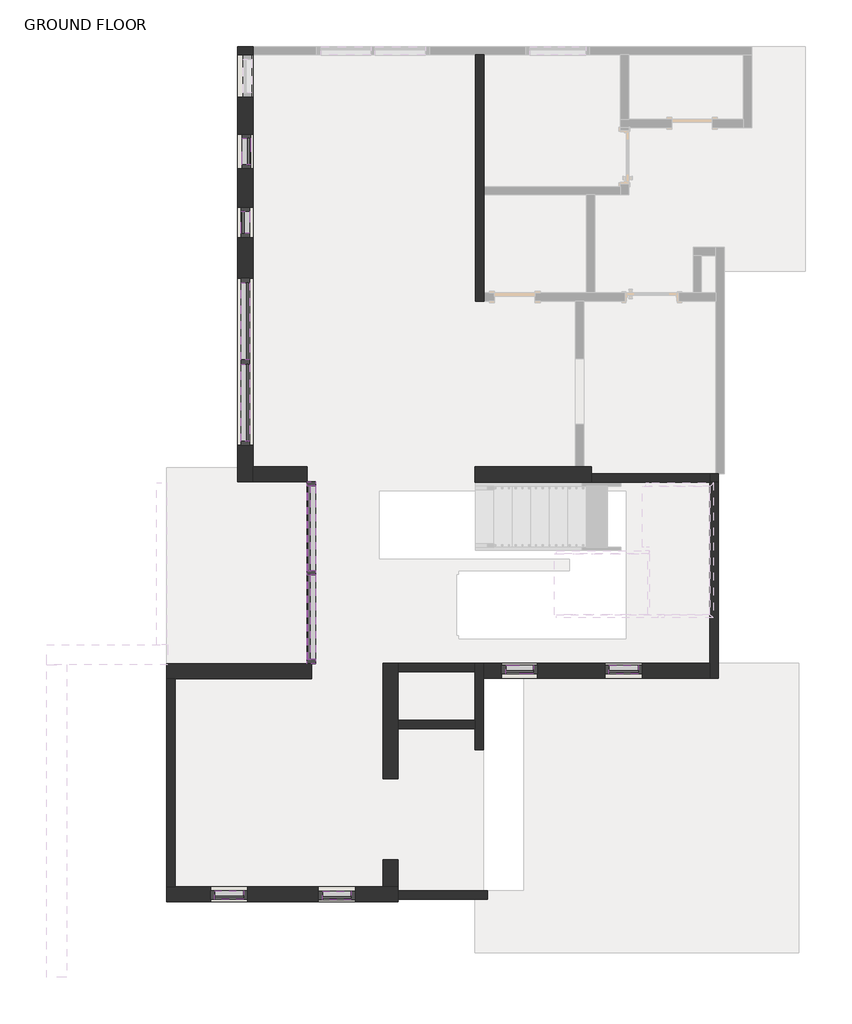
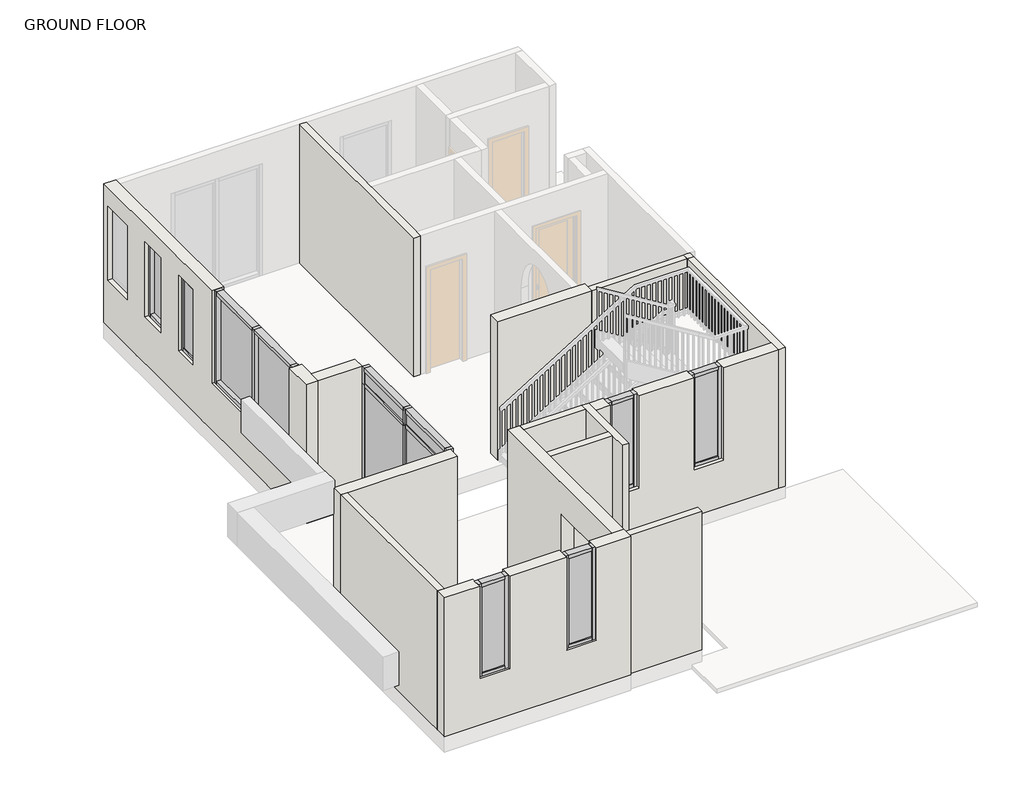
# One storey, part 1 of 3: 43 members, 16 walls, 12 plates.
"""IFC4 building model written with IfcOpenShell, lengths in millimetres."""

from ifc_helpers import new_model, si_unit, frame, origin, place, context, project, spatial, polyline, outline, extrude, faceted_brep, transform, mapped, element, save
from components import member_9ae880e2, member_2fc94954, member_ff9f2d30, member_7096a90e, member_6fb4a552, member_dc106669, member_69a911c1, member_2fae0574, member_d60e8053, member_28306602, member_d74100e1, member_f0fea5a5, member_f066cb84, member_ee409385, member_1c9aee36, member_0a8ab348, system_panel_glazed_1e1b7e15, system_panel_glazed_df80ca6a, system_panel_glazed_ba1f660c, system_panel_glazed_a5d4ee92, system_panel_glazed_c73a426b, system_panel_glazed_19c201ce, system_panel_glazed_de34110e, system_panel_glazed_f096bff0

model = new_model("IFC4")

# Units and contexts
model_context = context("Model", 3, world=origin())
ifc_project = project(units=[si_unit("LENGTHUNIT", "METRE", prefix="MILLI")], contexts=[model_context])

# Site, building, storey
site = spatial("IfcSite", under=ifc_project)
building = spatial("IfcBuilding", under=site)
storey = spatial("IfcBuildingStorey", under=building, Name="GROUND FLOOR", Elevation=304.8)

# Members
placement = place(None, origin())
member_shape = member_9ae880e2(model_context)
element("IfcMember", 1, ObjectType="Rectangular Mullion : 2.5\" x 5\" rectangular", at=placement, inside=storey, context=model_context, shape_type="MappedRepresentation", body=[
    mapped(member_shape, transform((-10742.5406521, -5304.9048674, 3048.0), x_axis=(0.0, 0.0, 1.0), y_axis=(1.0, 0.0, 0.0), z_axis=(0.0, 1.0, 0.0))),
])
element("IfcMember", 2, ObjectType="Rectangular Mullion : 2.5\" x 5\" rectangular", at=placement, inside=storey, context=model_context, shape_type="MappedRepresentation", body=[
    mapped(member_shape, transform((-10742.5406521, -6642.5105319, 3048.0), x_axis=(0.0, 0.0, 1.0), y_axis=(1.0, 0.0, 0.0), z_axis=(0.0, 1.0, 0.0))),
])
element("IfcMember", 3, ObjectType="Rectangular Mullion : 2.5\" x 5\" rectangular", at=placement, inside=storey, context=model_context, shape_type="MappedRepresentation", body=[
    mapped(member_shape, transform((-10742.5406521, -7916.6161964, 279.1402582), x_axis=(0.0, 0.0, -1.0), y_axis=(1.0, 0.0, 0.0), z_axis=(0.0, -1.0, 0.0))),
])
element("IfcMember", 4, ObjectType="Rectangular Mullion : 2.5\" x 5\" rectangular", at=placement, inside=storey, context=model_context, shape_type="MappedRepresentation", body=[
    mapped(member_shape, transform((-10742.5406521, -6579.0105319, 279.1402582), x_axis=(0.0, 0.0, -1.0), y_axis=(1.0, 0.0, 0.0), z_axis=(0.0, -1.0, 0.0))),
])
member_2_shape = member_2fc94954(model_context)
element("IfcMember", 5, ObjectType="Rectangular Mullion : 2.5\" x 5\" rectangular", at=placement, inside=storey, context=model_context, shape_type="MappedRepresentation", body=[
    mapped(member_2_shape, transform((-11735.5015106, -2244.2048674, 3048.0), x_axis=(0.0, 0.0, 1.0), y_axis=(1.0, 0.0, 0.0), z_axis=(0.0, 1.0, 0.0))),
])
element("IfcMember", 6, ObjectType="Rectangular Mullion : 2.5\" x 5\" rectangular", at=placement, inside=storey, context=model_context, shape_type="MappedRepresentation", body=[
    mapped(member_2_shape, transform((-11735.5015106, -3469.7548674, 3048.0), x_axis=(0.0, 0.0, 1.0), y_axis=(1.0, 0.0, 0.0), z_axis=(0.0, 1.0, 0.0))),
])
element("IfcMember", 7, ObjectType="Rectangular Mullion : 2.5\" x 5\" rectangular", at=placement, inside=storey, context=model_context, shape_type="MappedRepresentation", body=[
    mapped(member_2_shape, transform((-11735.5015106, -4631.8048674, 1219.2), x_axis=(0.0, 0.0, -1.0), y_axis=(1.0, 0.0, 0.0), z_axis=(0.0, -1.0, 0.0))),
])
element("IfcMember", 8, ObjectType="Rectangular Mullion : 2.5\" x 5\" rectangular", at=placement, inside=storey, context=model_context, shape_type="MappedRepresentation", body=[
    mapped(member_2_shape, transform((-11735.5015106, -3406.2548674, 1219.2), x_axis=(0.0, 0.0, -1.0), y_axis=(1.0, 0.0, 0.0), z_axis=(0.0, -1.0, 0.0))),
])
member_3_shape = member_ff9f2d30(model_context)
element("IfcMember", 9, ObjectType="Rectangular Mullion : 2.5\" x 5\" rectangular", at=placement, inside=storey, context=model_context, shape_type="MappedRepresentation", body=[
    mapped(member_3_shape, transform((-11735.5015106, -1171.7968948, 2709.2142793), x_axis=(0.0, 0.0, 1.0), y_axis=(1.0, 0.0, 0.0), z_axis=(0.0, 1.0, 0.0))),
])
element("IfcMember", 10, ObjectType="Rectangular Mullion : 2.5\" x 5\" rectangular", at=placement, inside=storey, context=model_context, shape_type="MappedRepresentation", body=[
    mapped(member_3_shape, transform((-11735.5015106, -1501.9968948, 1219.2), x_axis=(0.0, 0.0, -1.0), y_axis=(1.0, 0.0, 0.0), z_axis=(0.0, -1.0, 0.0))),
])
member_4_shape = member_7096a90e(model_context)
element("IfcMember", 11, ObjectType="Rectangular Mullion : 2.5\" x 5\" rectangular", at=placement, inside=storey, context=model_context, shape_type="MappedRepresentation", body=[
    mapped(member_4_shape, transform((-11716.8345465, -72.4462169, 2701.6314829), x_axis=(0.0, 0.0, 1.0), y_axis=(1.0, 0.0, 0.0), z_axis=(0.0, 1.0, 0.0))),
])
element("IfcMember", 12, ObjectType="Rectangular Mullion : 2.5\" x 5\" rectangular", at=placement, inside=storey, context=model_context, shape_type="MappedRepresentation", body=[
    mapped(member_4_shape, transform((-11716.8345465, -466.1462169, 1219.2), x_axis=(0.0, 0.0, -1.0), y_axis=(1.0, 0.0, 0.0), z_axis=(0.0, -1.0, 0.0))),
])
member_5_shape = member_6fb4a552(model_context)
element("IfcMember", 13, ObjectType="Rectangular Mullion : 2.5\" x 5\" rectangular", at=placement, inside=storey, context=model_context, shape_type="MappedRepresentation", body=[
    mapped(member_5_shape, transform((-6254.3081119, -8068.9864458, 3048.0), x_axis=(0.0, 0.0, 1.0), y_axis=(0.0, 1.0, 0.0), z_axis=(-1.0, 0.0, 0.0))),
])
element("IfcMember", 14, ObjectType="Rectangular Mullion : 2.5\" x 5\" rectangular", at=placement, inside=storey, context=model_context, shape_type="MappedRepresentation", body=[
    mapped(member_5_shape, transform((-5816.1581119, -8068.9864458, 1219.2), x_axis=(0.0, 0.0, -1.0), y_axis=(0.0, 1.0, 0.0), z_axis=(1.0, 0.0, 0.0))),
])
member_6_shape = member_dc106669(model_context)
element("IfcMember", 15, ObjectType="Rectangular Mullion : 2.5\" x 5\" rectangular", at=placement, inside=storey, context=model_context, shape_type="MappedRepresentation", body=[
    mapped(member_6_shape, transform((-7809.239759, -8066.9485269, 3048.0), x_axis=(0.0, 0.0, 1.0), y_axis=(0.0, 1.0, 0.0), z_axis=(-1.0, 0.0, 0.0))),
])
element("IfcMember", 16, ObjectType="Rectangular Mullion : 2.5\" x 5\" rectangular", at=placement, inside=storey, context=model_context, shape_type="MappedRepresentation", body=[
    mapped(member_6_shape, transform((-7396.489759, -8066.9485269, 1219.2), x_axis=(0.0, 0.0, -1.0), y_axis=(0.0, 1.0, 0.0), z_axis=(1.0, 0.0, 0.0))),
])
member_7_shape = member_69a911c1(model_context)
element("IfcMember", 17, ObjectType="Rectangular Mullion : 2.5\" x 5\" rectangular", at=placement, inside=storey, context=model_context, shape_type="MappedRepresentation", body=[
    mapped(member_7_shape, transform((-12196.3350942, -11462.667624, 3048.0), x_axis=(0.0, 0.0, 1.0), y_axis=(0.0, 1.0, 0.0), z_axis=(-1.0, 0.0, 0.0))),
])
element("IfcMember", 18, ObjectType="Rectangular Mullion : 2.5\" x 5\" rectangular", at=placement, inside=storey, context=model_context, shape_type="MappedRepresentation", body=[
    mapped(member_7_shape, transform((-10573.0486636, -11471.780526, 3048.0), x_axis=(0.0, 0.0, 1.0), y_axis=(0.0, 1.0, 0.0), z_axis=(-1.0, 0.0, 0.0))),
])
element("IfcMember", 19, ObjectType="Rectangular Mullion : 2.5\" x 5\" rectangular", at=placement, inside=storey, context=model_context, shape_type="MappedRepresentation", body=[
    mapped(member_7_shape, transform((-11764.5350942, -11462.667624, 1219.2), x_axis=(0.0, 0.0, -1.0), y_axis=(0.0, 1.0, 0.0), z_axis=(1.0, 0.0, 0.0))),
])
element("IfcMember", 20, ObjectType="Rectangular Mullion : 2.5\" x 5\" rectangular", at=placement, inside=storey, context=model_context, shape_type="MappedRepresentation", body=[
    mapped(member_7_shape, transform((-10141.2486636, -11471.780526, 1219.2), x_axis=(0.0, 0.0, -1.0), y_axis=(0.0, 1.0, 0.0), z_axis=(1.0, 0.0, 0.0))),
])
member_8_shape = member_2fae0574(model_context)
element("IfcMember", 21, ObjectType="Rectangular Mullion : 2.5\" x 5\" rectangular", at=placement, inside=storey, context=model_context, shape_type="MappedRepresentation", body=[
    mapped(member_8_shape, transform((-6317.8081119, -8068.9864458, 1219.2), x_axis=(-1.0, 0.0, 0.0), y_axis=(0.0, 1.0, 0.0), z_axis=(0.0, 0.0, -1.0))),
])
element("IfcMember", 22, ObjectType="Rectangular Mullion : 2.5\" x 5\" rectangular", at=placement, inside=storey, context=model_context, shape_type="MappedRepresentation", body=[
    mapped(member_8_shape, transform((-7872.739759, -8066.9485269, 1219.2), x_axis=(-1.0, 0.0, 0.0), y_axis=(0.0, 1.0, 0.0), z_axis=(0.0, 0.0, -1.0))),
])
element("IfcMember", 23, ObjectType="Rectangular Mullion : 2.5\" x 5\" rectangular", at=placement, inside=storey, context=model_context, shape_type="MappedRepresentation", body=[
    mapped(member_8_shape, transform((-12259.8350942, -11462.667624, 1219.2), x_axis=(-1.0, 0.0, 0.0), y_axis=(0.0, 1.0, 0.0), z_axis=(0.0, 0.0, -1.0))),
])
element("IfcMember", 24, ObjectType="Rectangular Mullion : 2.5\" x 5\" rectangular", at=placement, inside=storey, context=model_context, shape_type="MappedRepresentation", body=[
    mapped(member_8_shape, transform((-10636.5486636, -11471.780526, 1219.2), x_axis=(-1.0, 0.0, 0.0), y_axis=(0.0, 1.0, 0.0), z_axis=(0.0, 0.0, -1.0))),
])
element("IfcMember", 25, ObjectType="Rectangular Mullion : 2.5\" x 5\" rectangular", at=placement, inside=storey, context=model_context, shape_type="MappedRepresentation", body=[
    mapped(member_8_shape, transform((-5752.6581119, -8068.9864458, 3048.0), x_axis=(1.0, 0.0, 0.0), y_axis=(0.0, 1.0, 0.0), z_axis=(0.0, 0.0, 1.0))),
])
element("IfcMember", 26, ObjectType="Rectangular Mullion : 2.5\" x 5\" rectangular", at=placement, inside=storey, context=model_context, shape_type="MappedRepresentation", body=[
    mapped(member_8_shape, transform((-7332.989759, -8066.9485269, 3048.0), x_axis=(1.0, 0.0, 0.0), y_axis=(0.0, 1.0, 0.0), z_axis=(0.0, 0.0, 1.0))),
])
element("IfcMember", 27, ObjectType="Rectangular Mullion : 2.5\" x 5\" rectangular", at=placement, inside=storey, context=model_context, shape_type="MappedRepresentation", body=[
    mapped(member_8_shape, transform((-11701.0350942, -11462.667624, 3048.0), x_axis=(1.0, 0.0, 0.0), y_axis=(0.0, 1.0, 0.0), z_axis=(0.0, 0.0, 1.0))),
])
element("IfcMember", 28, ObjectType="Rectangular Mullion : 2.5\" x 5\" rectangular", at=placement, inside=storey, context=model_context, shape_type="MappedRepresentation", body=[
    mapped(member_8_shape, transform((-10077.7486636, -11471.780526, 3048.0), x_axis=(1.0, 0.0, 0.0), y_axis=(0.0, 1.0, 0.0), z_axis=(0.0, 0.0, 1.0))),
])
member_9_shape = member_d60e8053(model_context)
element("IfcMember", 29, ObjectType="Rectangular Mullion : 2.5\" x 5\" rectangular", at=placement, inside=storey, context=model_context, shape_type="MappedRepresentation", body=[
    mapped(member_9_shape, transform((-11735.5015106, -3438.0048674, 1219.2), x_axis=(0.0, 1.0, 0.0), y_axis=(1.0, 0.0, 0.0), z_axis=(0.0, 0.0, -1.0))),
])
element("IfcMember", 30, ObjectType="Rectangular Mullion : 2.5\" x 5\" rectangular", at=placement, inside=storey, context=model_context, shape_type="MappedRepresentation", body=[
    mapped(member_8_shape, transform((-11735.5015106, -2180.7048674, 1219.2), x_axis=(0.0, 1.0, 0.0), y_axis=(1.0, 0.0, 0.0), z_axis=(0.0, 0.0, -1.0))),
])
element("IfcMember", 31, ObjectType="Rectangular Mullion : 2.5\" x 5\" rectangular", at=placement, inside=storey, context=model_context, shape_type="MappedRepresentation", body=[
    mapped(member_8_shape, transform((-11735.5015106, -4695.3048674, 3048.0), x_axis=(0.0, -1.0, 0.0), y_axis=(1.0, 0.0, 0.0), z_axis=(0.0, 0.0, 1.0))),
])
member_10_shape = member_28306602(model_context)
element("IfcMember", 32, ObjectType="Rectangular Mullion : 2.5\" x 5\" rectangular", at=placement, inside=storey, context=model_context, shape_type="MappedRepresentation", body=[
    mapped(member_10_shape, transform((-11735.5015106, -1108.2968948, 1219.2), x_axis=(0.0, 1.0, 0.0), y_axis=(1.0, 0.0, 0.0), z_axis=(0.0, 0.0, -1.0))),
])
element("IfcMember", 33, ObjectType="Rectangular Mullion : 2.5\" x 5\" rectangular", at=placement, inside=storey, context=model_context, shape_type="MappedRepresentation", body=[
    mapped(member_10_shape, transform((-11735.5015106, -1565.4968948, 2709.2142793), x_axis=(0.0, -1.0, 0.0), y_axis=(1.0, 0.0, 0.0), z_axis=(0.0, 0.0, 1.0))),
])
member_11_shape = member_d74100e1(model_context)
element("IfcMember", 34, ObjectType="Rectangular Mullion : 2.5\" x 5\" rectangular", at=placement, inside=storey, context=model_context, shape_type="MappedRepresentation", body=[
    mapped(member_11_shape, transform((-11716.8345465, -8.9462169, 1219.2), x_axis=(0.0, 1.0, 0.0), y_axis=(1.0, 0.0, 0.0), z_axis=(0.0, 0.0, -1.0))),
])
element("IfcMember", 35, ObjectType="Rectangular Mullion : 2.5\" x 5\" rectangular", at=placement, inside=storey, context=model_context, shape_type="MappedRepresentation", body=[
    mapped(member_11_shape, transform((-11716.8345465, -529.6462169, 2701.6314829), x_axis=(0.0, -1.0, 0.0), y_axis=(1.0, 0.0, 0.0), z_axis=(0.0, 0.0, 1.0))),
])
member_12_shape = member_f0fea5a5(model_context)
element("IfcMember", 36, ObjectType="Rectangular Mullion : 2.5\" x 5\" rectangular", at=placement, inside=storey, context=model_context, shape_type="MappedRepresentation", body=[
    mapped(member_12_shape, transform((-10742.5406521, -6610.7605319, 279.1402582), x_axis=(0.0, 1.0, 0.0), y_axis=(1.0, 0.0, 0.0), z_axis=(0.0, 0.0, -1.0))),
])
member_13_shape = member_f066cb84(model_context)
element("IfcMember", 37, ObjectType="Rectangular Mullion : 2.5\" x 5\" rectangular", at=placement, inside=storey, context=model_context, shape_type="MappedRepresentation", body=[
    mapped(member_13_shape, transform((-10742.5406521, -6642.5105319, 2717.5402582), x_axis=(0.0, 0.0, 1.0), y_axis=(1.0, 0.0, 0.0), z_axis=(0.0, 1.0, 0.0))),
])
element("IfcMember", 38, ObjectType="Rectangular Mullion : 2.5\" x 5\" rectangular", at=placement, inside=storey, context=model_context, shape_type="MappedRepresentation", body=[
    mapped(member_13_shape, transform((-10742.5406521, -5304.9048674, 2717.5402582), x_axis=(0.0, 0.0, 1.0), y_axis=(1.0, 0.0, 0.0), z_axis=(0.0, 1.0, 0.0))),
])
member_14_shape = member_ee409385(model_context)
element("IfcMember", 39, ObjectType="Rectangular Mullion : 2.5\" x 5\" rectangular", at=placement, inside=storey, context=model_context, shape_type="MappedRepresentation", body=[
    mapped(member_14_shape, transform((-10742.5406521, -5241.4048674, 279.1402582), x_axis=(0.0, 1.0, 0.0), y_axis=(1.0, 0.0, 0.0), z_axis=(0.0, 0.0, -1.0))),
])
element("IfcMember", 40, ObjectType="Rectangular Mullion : 2.5\" x 5\" rectangular", at=placement, inside=storey, context=model_context, shape_type="MappedRepresentation", body=[
    mapped(member_14_shape, transform((-10742.5406521, -7980.1161964, 2717.5402582), x_axis=(0.0, -1.0, 0.0), y_axis=(1.0, 0.0, 0.0), z_axis=(0.0, 0.0, 1.0))),
])
member_15_shape = member_1c9aee36(model_context)
element("IfcMember", 41, ObjectType="Rectangular Mullion : 2.5\" x 5\" rectangular", at=placement, inside=storey, context=model_context, shape_type="MappedRepresentation", body=[
    mapped(member_15_shape, transform((-10742.5406521, -6610.7605319, 2717.5402582), x_axis=(0.0, 1.0, 0.0), y_axis=(1.0, 0.0, 0.0), z_axis=(0.0, 0.0, -1.0))),
])
member_16_shape = member_0a8ab348(model_context)
element("IfcMember", 42, ObjectType="Rectangular Mullion : 2.5\" x 5\" rectangular", at=placement, inside=storey, context=model_context, shape_type="MappedRepresentation", body=[
    mapped(member_16_shape, transform((-10742.5406521, -7980.1161964, 3048.0), x_axis=(0.0, -1.0, 0.0), y_axis=(1.0, 0.0, 0.0), z_axis=(0.0, 0.0, 1.0))),
])
element("IfcMember", 43, ObjectType="Rectangular Mullion : 2.5\" x 5\" rectangular", at=placement, inside=storey, context=model_context, shape_type="MappedRepresentation", body=[
    mapped(member_16_shape, transform((-10742.5406521, -5241.4048674, 2717.5402582), x_axis=(0.0, 1.0, 0.0), y_axis=(1.0, 0.0, 0.0), z_axis=(0.0, 0.0, -1.0))),
])

# Plates
system_panel_glazed_shape = system_panel_glazed_1e1b7e15(model_context)
element("IfcPlate", 44, ObjectType="System Panel : Glazed", at=placement, inside=storey, context=model_context, shape_type="MappedRepresentation", body=[
    mapped(system_panel_glazed_shape, transform((-11735.5015106, -4050.7798674, 1282.7), x_axis=(0.0, 1.0, 0.0), y_axis=(-1.0, 0.0, 0.0), z_axis=(0.0, 0.0, 1.0))),
])
element("IfcPlate", 45, ObjectType="System Panel : Glazed", at=placement, inside=storey, context=model_context, shape_type="MappedRepresentation", body=[
    mapped(system_panel_glazed_shape, transform((-11735.5015106, -2825.2298674, 1282.7), x_axis=(0.0, 1.0, 0.0), y_axis=(-1.0, 0.0, 0.0), z_axis=(0.0, 0.0, 1.0))),
])
system_panel_glazed_2_shape = system_panel_glazed_df80ca6a(model_context)
element("IfcPlate", 46, ObjectType="System Panel : Glazed", at=placement, inside=storey, context=model_context, shape_type="MappedRepresentation", body=[
    mapped(system_panel_glazed_2_shape, transform((-11735.5015106, -1336.8968948, 1282.7), x_axis=(0.0, 1.0, 0.0), y_axis=(-1.0, 0.0, 0.0), z_axis=(0.0, 0.0, 1.0))),
])
system_panel_glazed_3_shape = system_panel_glazed_ba1f660c(model_context)
element("IfcPlate", 47, ObjectType="System Panel : Glazed", at=placement, inside=storey, context=model_context, shape_type="MappedRepresentation", body=[
    mapped(system_panel_glazed_3_shape, transform((-11716.8345465, -269.2962169, 1282.7), x_axis=(0.0, 1.0, 0.0), y_axis=(-1.0, 0.0, 0.0), z_axis=(0.0, 0.0, 1.0))),
])
system_panel_glazed_4_shape = system_panel_glazed_a5d4ee92(model_context)
element("IfcPlate", 48, ObjectType="System Panel : Glazed", at=placement, inside=storey, context=model_context, shape_type="MappedRepresentation", body=[
    mapped(system_panel_glazed_4_shape, transform((-6035.2331119, -8068.9864458, 1282.7), x_axis=(-1.0, 0.0, 0.0), y_axis=(0.0, -1.0, 0.0), z_axis=(0.0, 0.0, 1.0))),
])
system_panel_glazed_5_shape = system_panel_glazed_c73a426b(model_context)
element("IfcPlate", 49, ObjectType="System Panel : Glazed", at=placement, inside=storey, context=model_context, shape_type="MappedRepresentation", body=[
    mapped(system_panel_glazed_5_shape, transform((-7602.864759, -8066.9485269, 1282.7), x_axis=(-1.0, 0.0, 0.0), y_axis=(0.0, -1.0, 0.0), z_axis=(0.0, 0.0, 1.0))),
])
system_panel_glazed_6_shape = system_panel_glazed_19c201ce(model_context)
element("IfcPlate", 50, ObjectType="System Panel : Glazed", at=placement, inside=storey, context=model_context, shape_type="MappedRepresentation", body=[
    mapped(system_panel_glazed_6_shape, transform((-11980.4350942, -11462.667624, 1282.7), x_axis=(-1.0, 0.0, 0.0), y_axis=(0.0, -1.0, 0.0), z_axis=(0.0, 0.0, 1.0))),
])
element("IfcPlate", 51, ObjectType="System Panel : Glazed", at=placement, inside=storey, context=model_context, shape_type="MappedRepresentation", body=[
    mapped(system_panel_glazed_6_shape, transform((-10357.1486636, -11471.780526, 1282.7), x_axis=(-1.0, 0.0, 0.0), y_axis=(0.0, -1.0, 0.0), z_axis=(0.0, 0.0, 1.0))),
])
system_panel_glazed_7_shape = system_panel_glazed_de34110e(model_context)
element("IfcPlate", 52, ObjectType="System Panel : Glazed", at=placement, inside=storey, context=model_context, shape_type="MappedRepresentation", body=[
    mapped(system_panel_glazed_7_shape, transform((-10742.5406521, -7279.5633642, 342.6402582), x_axis=(0.0, 1.0, 0.0), y_axis=(-1.0, 0.0, 0.0), z_axis=(0.0, 0.0, 1.0))),
])
element("IfcPlate", 53, ObjectType="System Panel : Glazed", at=placement, inside=storey, context=model_context, shape_type="MappedRepresentation", body=[
    mapped(system_panel_glazed_7_shape, transform((-10742.5406521, -5941.9576997, 342.6402582), x_axis=(0.0, 1.0, 0.0), y_axis=(-1.0, 0.0, 0.0), z_axis=(0.0, 0.0, 1.0))),
])
system_panel_glazed_8_shape = system_panel_glazed_f096bff0(model_context)
element("IfcPlate", 54, ObjectType="System Panel : Glazed", at=placement, inside=storey, context=model_context, shape_type="MappedRepresentation", body=[
    mapped(system_panel_glazed_8_shape, transform((-10742.5406521, -7279.5633642, 2749.2902582), x_axis=(0.0, 1.0, 0.0), y_axis=(-1.0, 0.0, 0.0), z_axis=(0.0, 0.0, 1.0))),
])
element("IfcPlate", 55, ObjectType="System Panel : Glazed", at=placement, inside=storey, context=model_context, shape_type="MappedRepresentation", body=[
    mapped(system_panel_glazed_8_shape, transform((-10742.5406521, -5941.9576997, 2749.2902582), x_axis=(0.0, 1.0, 0.0), y_axis=(-1.0, 0.0, 0.0), z_axis=(0.0, 0.0, 1.0))),
])

# Walls
element("IfcWall", 56, ObjectType="EXTERIOR WALL 9\"", at=placement, inside=storey, context=model_context, shape_type="Brep", body=[
    faceted_brep([(-12920.5906521, -11568.2453012, 304.8), (-9433.822653, -11568.2453012, 304.8), (-9433.822653, -11568.2453012, 3048.0), (-10077.7486636, -11568.2453012, 3048.0), (-10077.7486636, -11568.2453012, 1219.2), (-10636.5486636, -11568.2453012, 1219.2), (-10636.5486636, -11568.2453012, 3048.0), (-11701.0350942, -11568.2453012, 3048.0), (-11701.0350942, -11568.2453012, 1219.2), (-12259.8350942, -11568.2453012, 1219.2), (-12259.8350942, -11568.2453012, 3048.0), (-12920.5906521, -11568.2453012, 3048.0), (-9433.822653, -11339.6453012, 304.8), (-9662.422653, -11339.6453012, 304.8), (-12793.5906521, -11339.6453012, 304.8), (-12920.5906521, -11339.6453012, 304.8), (-12920.5906521, -11339.6453012, 3048.0), (-12793.5906521, -11339.6453012, 3048.0), (-12259.8350942, -11339.6453012, 3048.0), (-12259.8350942, -11339.6453012, 1219.2), (-11701.0350942, -11339.6453012, 1219.2), (-11701.0350942, -11339.6453012, 3048.0), (-10636.5486636, -11339.6453012, 3048.0), (-10636.5486636, -11339.6453012, 1219.2), (-10077.7486636, -11339.6453012, 1219.2), (-10077.7486636, -11339.6453012, 3048.0), (-9662.422653, -11339.6453012, 3048.0), (-9433.822653, -11339.6453012, 3048.0), (-9433.822653, -11403.1453012, 304.8), (-9433.822653, -11530.1453012, 304.8), (-9433.822653, -11530.1453012, 3048.0), (-9433.822653, -11403.1453012, 3048.0)], [[[0, 1, 2, 3, 4, 5, 6, 7, 8, 9, 10, 11]], [[12, 13, 14, 15, 16, 17, 18, 19, 20, 21, 22, 23, 24, 25, 26, 27]], [[1, 0, 15, 14, 13, 12, 28, 29]], [[16, 11, 10, 18, 17]], [[2, 30, 31, 27, 26, 25, 3]], [[21, 7, 6, 22]], [[2, 1, 29, 28, 12, 27, 31, 30]], [[0, 11, 16, 15]], [[20, 8, 7, 21]], [[9, 19, 18, 10]], [[8, 20, 19, 9]], [[24, 4, 3, 25]], [[5, 23, 22, 6]], [[4, 24, 23, 5]]]),
])
element("IfcWall", 57, ObjectType="EXTERIOR WALL 9\"", at=placement, inside=storey, context=model_context, shape_type="Brep", body=[
    faceted_brep([(-9433.822653, -7975.1830995, 3048.0), (-9433.822653, -8102.1830995, 3048.0), (-9433.822653, -8831.0161964, 3048.0), (-9433.822653, -8958.0161964, 3048.0), (-9433.822653, -11339.6453012, 3048.0), (-9433.822653, -11339.6453012, 304.8), (-9433.822653, -10933.2453012, 304.8), (-9433.822653, -10933.2453012, 2438.4), (-9433.822653, -9714.0453012, 2438.4), (-9433.822653, -9714.0453012, 304.8), (-9433.822653, -8958.0161964, 304.8), (-9433.822653, -8831.0161964, 304.8), (-9433.822653, -8102.1830995, 304.8), (-9433.822653, -7975.1830995, 304.8), (-9662.422653, -11339.6453012, 3048.0), (-9662.422653, -7975.1830995, 3048.0), (-9662.422653, -7975.1830995, 304.8), (-9662.422653, -9714.0453012, 304.8), (-9662.422653, -9714.0453012, 2438.4), (-9662.422653, -10933.2453012, 2438.4), (-9662.422653, -10933.2453012, 304.8), (-9662.422653, -11339.6453012, 304.8)], [[[0, 1, 2, 3, 4, 5, 6, 7, 8, 9, 10, 11, 12, 13]], [[14, 15, 16, 17, 18, 19, 20, 21]], [[5, 21, 20, 6]], [[16, 13, 12, 11, 10, 9, 17]], [[4, 3, 2, 1, 0, 15, 14]], [[5, 4, 14, 21]], [[0, 13, 16, 15]], [[19, 7, 6, 20]], [[7, 19, 18, 8]], [[8, 18, 17, 9]]]),
])
element("IfcWall", 58, ObjectType="EXTERIOR WALL 9\"", at=placement, inside=storey, context=model_context, shape_type="Brep", body=[
    faceted_brep([(-11849.8015106, 1311.7951326, 304.8), (-11849.8015106, -5241.4048674, 304.8), (-11849.8015106, -5241.4048674, 3048.0), (-11849.8015106, -4695.3048674, 3048.0), (-11849.8015106, -4695.3048674, 1219.2), (-11849.8015106, -2180.7048674, 1219.2), (-11849.8015106, -2180.7048674, 3048.0), (-11849.8015106, 1311.7951326, 3048.0), (-11849.8015106, -1565.4968948, 2709.2142793), (-11849.8015106, -1565.4968948, 1219.2), (-11849.8015106, -1108.2968948, 1219.2), (-11849.8015106, -1108.2968948, 2709.2142793), (-11849.8015106, -529.6462169, 2701.6314829), (-11849.8015106, -529.6462169, 1219.2), (-11849.8015106, -8.9462169, 1219.2), (-11849.8015106, -8.9462169, 2701.6314829), (-11849.8015106, 550.8802108, 2682.3285226), (-11849.8015106, 550.8802108, 1219.2), (-11849.8015106, 1184.7951326, 1219.2), (-11849.8015106, 1184.7951326, 2682.3285226), (-11621.2015106, -5241.4048674, 304.8), (-11621.2015106, -5012.8048674, 304.8), (-11621.2015106, 1184.7951326, 304.8), (-11621.2015106, 1311.7951326, 304.8), (-11621.2015106, 1311.7951326, 3048.0), (-11621.2015106, 1184.7951326, 3048.0), (-11621.2015106, -2180.7048674, 3048.0), (-11621.2015106, -2180.7048674, 1219.2), (-11621.2015106, -4695.3048674, 1219.2), (-11621.2015106, -4695.3048674, 3048.0), (-11621.2015106, -5012.8048674, 3048.0), (-11621.2015106, -5241.4048674, 3048.0), (-11621.2015106, -1565.4968948, 1219.2), (-11621.2015106, -1565.4968948, 2709.2142793), (-11621.2015106, -1108.2968948, 2709.2142793), (-11621.2015106, -1108.2968948, 1219.2), (-11621.2015106, -529.6462169, 1219.2), (-11621.2015106, -529.6462169, 2701.6314829), (-11621.2015106, -8.9462169, 2701.6314829), (-11621.2015106, -8.9462169, 1219.2), (-11621.2015106, 550.8802108, 1219.2), (-11621.2015106, 550.8802108, 2682.3285226), (-11621.2015106, 1184.7951326, 2682.3285226), (-11621.2015106, 1184.7951326, 1219.2)], [[[0, 1, 2, 3, 4, 5, 6, 7], [8, 9, 10, 11], [12, 13, 14, 15], [16, 17, 18, 19]], [[20, 21, 22, 23, 24, 25, 26, 27, 28, 29, 30, 31], [32, 33, 34, 35], [36, 37, 38, 39], [40, 41, 42, 43]], [[1, 0, 23, 22, 21, 20]], [[2, 31, 30, 29, 3]], [[24, 7, 6, 26, 25]], [[2, 1, 20, 31]], [[0, 7, 24, 23]], [[28, 4, 3, 29]], [[5, 27, 26, 6]], [[4, 28, 27, 5]], [[32, 9, 8, 33]], [[33, 8, 11, 34]], [[34, 11, 10, 35]], [[9, 32, 35, 10]], [[12, 37, 36, 13]], [[37, 12, 15, 38]], [[38, 15, 14, 39]], [[13, 36, 39, 14]], [[16, 41, 40, 17]], [[41, 16, 19, 42]], [[42, 19, 18, 43]], [[17, 40, 43, 18]]]),
])
element("IfcWall", 59, ObjectType="EXTERIOR WALL 9\"", at=placement, inside=storey, context=model_context, shape_type="SweptSolid", body=[
    extrude(outline(polyline([(-10806.0406521, -5241.4048674), (-11621.2015106, -5241.4048674), (-11621.2015106, -5012.8048674), (-10806.0406521, -5012.8048674), (-10806.0406521, -5241.4048674)])), frame((0.0, 0.0, 304.8), z_axis=(0.0, 0.0, 1.0), x_axis=(1.0, 0.0, 0.0)), (0.0, 0.0, 1.0), 2743.2),
])
element("IfcWall", 60, ObjectType="EXTERIOR WALL 9\"", at=placement, inside=storey, context=model_context, shape_type="Brep", body=[
    faceted_brep([(-12920.5906521, -8208.7161964, 304.8), (-12793.5906521, -8208.7161964, 304.8), (-10736.1906521, -8208.7161964, 304.8), (-10736.1906521, -8208.7161964, 3048.0), (-12793.5906521, -8208.7161964, 3048.0), (-12920.5906521, -8208.7161964, 3048.0), (-12920.5906521, -7980.1161964, 304.8), (-12920.5906521, -7980.1161964, 3048.0), (-10869.5406521, -7980.1161964, 3048.0), (-10742.5406521, -7980.1161964, 3048.0), (-10736.1906521, -7980.1161964, 3048.0), (-10736.1906521, -7980.1161964, 304.8), (-10742.5406521, -7980.1161964, 304.8), (-10869.5406521, -7980.1161964, 304.8)], [[[0, 1, 2, 3, 4, 5]], [[6, 7, 8, 9, 10, 11, 12, 13]], [[2, 1, 0, 6, 13, 12, 11]], [[3, 2, 11, 10]], [[5, 4, 3, 10, 9, 8, 7]], [[0, 5, 7, 6]]]),
])
element("IfcWall", 61, ObjectType="EXTERIOR WALL 9\"", at=placement, inside=storey, context=model_context, shape_type="SweptSolid", body=[
    extrude(outline(polyline([(304.8, -8147.3960918), (304.8, -4732.5727979), (3048.0, -4732.5727979), (3048.0, -5752.6581119), (1219.2, -5752.6581119), (1219.2, -6317.8081119), (3048.0, -6317.8081119), (3048.0, -7332.989759), (1219.2, -7332.989759), (1219.2, -7872.739759), (3048.0, -7872.739759), (3048.0, -8147.3960918), (304.8, -8147.3960918)])), frame((0.0, -8203.7830995, 0.0), z_axis=(0.0, 1.0, 0.0), x_axis=(0.0, 0.0, 1.0)), (0.0, 0.0, 1.0), 228.6),
])
element("IfcWall", 62, ObjectType="EXTERIOR WALL 9\"", at=placement, inside=storey, context=model_context, shape_type="Brep", body=[
    faceted_brep([(-8271.0210191, -5246.8337491, 304.8), (-6518.4210191, -5246.8337491, 304.8), (-6518.4210191, -5246.8337491, 3048.0), (-8271.0210191, -5246.8337491, 3048.0), (-8271.0210191, -5018.2337491, 304.8), (-8271.0210191, -5018.2337491, 3048.0), (-6758.2911408, -5018.2337491, 3048.0), (-6631.2911408, -5018.2337491, 3048.0), (-6518.4210191, -5018.2337491, 3048.0), (-6518.4210191, -5018.2337491, 304.8), (-6631.2911408, -5018.2337491, 304.8), (-6758.2911408, -5018.2337491, 304.8), (-6518.4210191, -5119.8337491, 304.8), (-6518.4210191, -5119.8337491, 3048.0)], [[[0, 1, 2, 3]], [[4, 5, 6, 7, 8, 9, 10, 11]], [[1, 0, 4, 11, 10, 9, 12]], [[2, 1, 12, 9, 8, 13]], [[3, 2, 13, 8, 7, 6, 5]], [[0, 3, 5, 4]]]),
])
element("IfcWall", 63, ObjectType="INTERIOR WALL PAINT 5\"", at=placement, inside=storey, context=model_context, shape_type="Brep", body=[
    faceted_brep([(-8269.5911408, 1184.7951326, 304.8), (-8269.5911408, -2523.6048674, 304.8), (-8269.5911408, -2523.6048674, 3048.0), (-8269.5911408, 1184.7951326, 3048.0), (-8142.5911408, 1184.7951326, 304.8), (-8142.5911408, 1184.7951326, 3048.0), (-8142.5911408, -796.4048674, 3048.0), (-8142.5911408, -923.4048674, 3048.0), (-8142.5911408, -2396.6048674, 3048.0), (-8142.5911408, -2523.6048674, 3048.0), (-8142.5911408, -2523.6048674, 304.8), (-8142.5911408, -2396.6048674, 304.8), (-8142.5911408, -923.4048674, 304.8), (-8142.5911408, -796.4048674, 304.8)], [[[0, 1, 2, 3]], [[4, 5, 6, 7, 8, 9, 10, 11, 12, 13]], [[1, 0, 4, 13, 12, 11, 10]], [[3, 2, 9, 8, 7, 6, 5]], [[0, 3, 5, 4]], [[2, 1, 10, 9]]]),
])
element("IfcWall", 64, ObjectType="INTERIOR WALL PAINT 5\"", at=placement, inside=storey, context=model_context, shape_type="SweptSolid", body=[
    extrude(outline(polyline([(-12920.5906521, -11339.6453012), (-12920.5906521, -8208.7161964), (-12793.5906521, -8208.7161964), (-12793.5906521, -11339.6453012), (-12920.5906521, -11339.6453012)])), frame((0.0, 0.0, 304.8), z_axis=(0.0, 0.0, 1.0), x_axis=(1.0, 0.0, 0.0)), (0.0, 0.0, 1.0), 2743.2),
])
element("IfcWall", 65, ObjectType="INTERIOR WALL PAINT 5\"", at=placement, inside=storey, context=model_context, shape_type="Brep", body=[
    faceted_brep([(-4605.5727979, -8203.7830995, 304.8), (-4605.5727979, -5246.8337491, 304.8), (-4605.5727979, -5246.8337491, 3048.0), (-4605.5727979, -8203.7830995, 3048.0), (-4732.5727979, -8203.7830995, 304.8), (-4732.5727979, -8203.7830995, 3048.0), (-4732.5727979, -7975.1830995, 3048.0), (-4732.5727979, -5246.8337491, 3048.0), (-4732.5727979, -5246.8337491, 304.8), (-4732.5727979, -7975.1830995, 304.8)], [[[0, 1, 2, 3]], [[4, 5, 6, 7, 8, 9]], [[1, 0, 4, 9, 8]], [[3, 2, 7, 6, 5]], [[0, 3, 5, 4]], [[2, 1, 8, 7]]]),
])
element("IfcWall", 66, ObjectType="INTERIOR WALL PAINT 5\"", at=placement, inside=storey, context=model_context, shape_type="SweptSolid", body=[
    extrude(outline(polyline([(-6518.4210191, -5119.8337491), (-4733.1514303, -5119.8337491), (-4733.1514303, -5246.8337491), (-6518.4210191, -5246.8337491), (-6518.4210191, -5119.8337491)])), frame((0.0, 0.0, 304.8), z_axis=(0.0, 0.0, 1.0), x_axis=(1.0, 0.0, 0.0)), (0.0, 0.0, 1.0), 2743.2),
])
element("IfcWall", 67, ObjectType="INTERIOR WALL PAINT 5\"", at=placement, inside=storey, context=model_context, shape_type="Brep", body=[
    faceted_brep([(-4733.1514303, -5246.8337491, 304.8), (-4732.5727979, -5246.8337491, 304.8), (-4605.5727979, -5246.8337491, 304.8), (-4605.5727979, -5246.8337491, 3048.0), (-4732.5727979, -5246.8337491, 3048.0), (-4733.1514303, -5246.8337491, 3048.0), (-4733.1514303, -5119.8337491, 304.8), (-4733.1514303, -5119.8337491, 3048.0), (-4643.6727979, -5119.8337491, 3048.0), (-4605.5727979, -5119.8337491, 3048.0), (-4605.5727979, -5119.8337491, 304.8), (-4643.6727979, -5119.8337491, 304.8)], [[[0, 1, 2, 3, 4, 5]], [[6, 7, 8, 9, 10, 11]], [[2, 1, 0, 6, 11, 10]], [[5, 4, 3, 9, 8, 7]], [[0, 5, 7, 6]], [[3, 2, 10, 9]]]),
])
element("IfcWall", 68, ObjectType="INTERIOR WALL PAINT 5\"", at=placement, inside=storey, context=model_context, shape_type="SweptSolid", body=[
    extrude(outline(polyline([(-8274.3960918, -8958.0161964), (-9433.822653, -8958.0161964), (-9433.822653, -8831.0161964), (-8274.3960918, -8831.0161964), (-8274.3960918, -8958.0161964)])), frame((0.0, 0.0, 304.8), z_axis=(0.0, 0.0, 1.0), x_axis=(1.0, 0.0, 0.0)), (0.0, 0.0, 1.0), 2743.2),
])
element("IfcWall", 69, ObjectType="INTERIOR WALL PAINT 5\"", at=placement, inside=storey, context=model_context, shape_type="Brep", body=[
    faceted_brep([(-8147.3960918, -9276.1338719, 304.8), (-8147.3960918, -8203.7830995, 304.8), (-8147.3960918, -7975.1830995, 304.8), (-8147.3960918, -7975.1830995, 3048.0), (-8147.3960918, -8203.7830995, 3048.0), (-8147.3960918, -9276.1338719, 3048.0), (-8274.3960918, -9276.1338719, 304.8), (-8274.3960918, -9276.1338719, 3048.0), (-8274.3960918, -8958.0161964, 3048.0), (-8274.3960918, -8831.0161964, 3048.0), (-8274.3960918, -8102.1830995, 3048.0), (-8274.3960918, -7975.1830995, 3048.0), (-8274.3960918, -7975.1830995, 304.8), (-8274.3960918, -8102.1830995, 304.8), (-8274.3960918, -8831.0161964, 304.8), (-8274.3960918, -8958.0161964, 304.8)], [[[0, 1, 2, 3, 4, 5]], [[6, 7, 8, 9, 10, 11, 12, 13, 14, 15]], [[2, 1, 0, 6, 15, 14, 13, 12]], [[5, 4, 3, 11, 10, 9, 8, 7]], [[0, 5, 7, 6]], [[3, 2, 12, 11]]]),
])
element("IfcWall", 70, ObjectType="INTERIOR WALL PAINT 5\"", at=placement, inside=storey, context=model_context, shape_type="SweptSolid", body=[
    extrude(outline(polyline([(-8087.622653, -11530.1453012), (-9433.822653, -11530.1453012), (-9433.822653, -11403.1453012), (-8087.622653, -11403.1453012), (-8087.622653, -11530.1453012)])), frame((0.0, 0.0, 304.8), z_axis=(0.0, 0.0, 1.0), x_axis=(1.0, 0.0, 0.0)), (0.0, 0.0, 1.0), 2743.2),
])
element("IfcWall", 71, ObjectType="INTERIOR WALL PAINT 5\"", at=placement, inside=storey, context=model_context, shape_type="SweptSolid", body=[
    extrude(outline(polyline([(-9433.822653, -7975.1830995), (-8274.3960918, -7975.1830995), (-8274.3960918, -8102.1830995), (-9433.822653, -8102.1830995), (-9433.822653, -7975.1830995)])), frame((0.0, 0.0, 304.8), z_axis=(0.0, 0.0, 1.0), x_axis=(1.0, 0.0, 0.0)), (0.0, 0.0, 1.0), 2743.2),
])

save(model, "model.ifc")

# Revit data of these elements
# Type "Rectangular Mullion : 2.5\" x 5\" rectangular"
#   built-in parameter 1007304 = 0.416667 (stored number, unit not read)
#   built-in parameter 1007301 = 0.104167 (stored number, unit not read)
#   built-in parameter 1007300 = 0.104167 (stored number, unit not read)
# Type "System Panel : Glazed"
#   Construction Type Id = "GSP4R"
#   Analytic Construction = "1/8 in Pilkington single glazing"
#   Visual Light Transmittance = 0.9
#   Solar Heat Gain Coefficient = 0.86
#   Heat Transfer Coefficient (U) = 1.18115 BTU/(h·ft²·°F)
#   Define Thermal Properties by = 1
# Type "EXTERIOR WALL 9\""
#   Assembly Code = "B2010"
#   Layers, outside or top first: 0' - 9" "EXTERIOR WALL PAINT" (function 1)
# Type "INTERIOR WALL PAINT 5\""
#   Assembly Code = "B2010"
#   Layers, outside or top first: 0' - 5" "EXTERIOR WALL PAINT" (function 1)
# Elements 1, 2, 3, 4, 5, 6, 7, 8, 9, 10, 11, 12, 13, 14, 15, 16, 17, 18, 19, 20, 21, 22, 23, 24, 25, 26, 27, 28, 29, 30, 31, 32, 33, 34, 35, 36, 37, 38, 39, 40, 41, 42, 43 (IfcMember, "Rectangular Mullion : 2.5\" x 5\" rectangular")
#   Phase Created = New Construction
# Elements 44, 45, 46, 47, 48, 49, 50, 51, 52, 53, 54, 55 (IfcPlate, "System Panel : Glazed")
#   Phase Created = New Construction
#   Materials on its faces: "Glass"
# Elements 56, 57, 58, 59, 60, 61, 62 (IfcWall, "EXTERIOR WALL 9\"")
#   Top Offset = 0' - 0"
#   Base Offset = 0' - 0"
#   wall height = 9' - 0"
#   Phase Created = New Construction
#   Base Constraint = GROUND FLOOR
#   Top Constraint = FIRST FLR
#   Materials on its faces: "EXTERIOR WALL PAINT"
# Elements 63, 64, 65, 66, 67, 68, 69, 70, 71 (IfcWall, "INTERIOR WALL PAINT 5\"")
#   Top Offset = 0' - 0"
#   Base Offset = 0' - 0"
#   wall height = 9' - 0"
#   Phase Created = New Construction
#   Base Constraint = GROUND FLOOR
#   Top Constraint = FIRST FLR
#   Materials on its faces: "EXTERIOR WALL PAINT"
# Materials
#   "EXTERIOR WALL PAINT": class "Generic", colour RGB 120 120 120, transparency 0, Cost = 0
#   "Glass": class "Glass", colour RGB 0 128 192, transparency 0.75, Description = "Soda Lime Glass", Cost = 0
# Room at (-5093.402, 702.195) mm, phase "New Construction", upper level "GROUND FLOOR", upper offset 10' - 0", lower offset 0' - 0"
#   Number = "1"
#   Name = "WASH"
# Room at (-7367.891, -1660.005) mm, phase "New Construction", upper level "GROUND FLOOR", upper offset 10' - 0", lower offset 0' - 0"
#   Number = "2"
#   Name = "TOILET"
# Room at (-7113.296, 194.195) mm, phase "New Construction", upper level "GROUND FLOOR", upper offset 10' - 0", lower offset 0' - 0"
#   Number = "3"
#   Name = "BATH"
# Room at (-4752.386, -2117.559) mm, phase "New Construction", upper level "GROUND FLOOR", upper offset 10' - 0", lower offset 0' - 0"
#   Number = "4"
#   Name = "KITCHEN"
# Room at (-8879.509, -8466.6) mm, phase "New Construction", upper level "GROUND FLOOR", upper offset 10' - 0", lower offset 0' - 0"
#   Number = "5"
#   Name = "BATH"
# Room at (-8718.632, -5102.825) mm, phase "New Construction", upper level "GROUND FLOOR", upper offset 10' - 0", lower offset 0' - 0"
#   Number = "6"
#   Name = "LIVING ROOM AND DINING ROOM"
